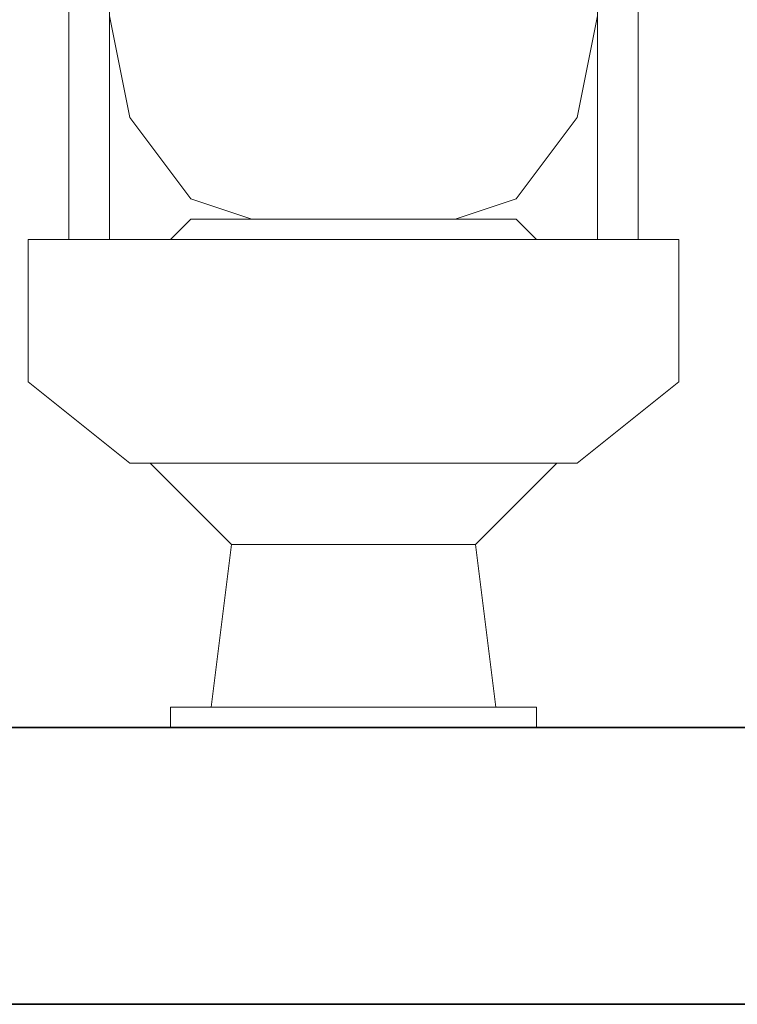
# Model space of a CAD drawing. Units: inches. Extents: x 64 to 1167, y 117 to 939.
# Tile 33 of 56: x 1051 to 1074, y 428 to 460. Entities that reach past the tile are written whole.
import ezdxf

# ---------------------------------------------------------------- set-up
doc = ezdxf.new("R2010")
doc.units = ezdxf.units.IN
doc.header["$MEASUREMENT"] = 0
doc.layers.add('A-FLOR-FIXT', color=8, linetype='Continuous', lineweight=18)
doc.layers.add('A-SECT', color=7, linetype='Continuous', lineweight=35)

# ---------------------------------------------------------------- blocks, each defined once
blk = doc.blocks.new('A$C02040E19')
for p, q in [((33.6, 403.2, 10), (33.6, 789.6, 10)), ((33.6, 403.2, 10), (33.6, 789.6, 10)), ((67.2, 789.6, 10), (67.2, 403.2, 10)), ((470.4, 789.6, 10), (470.4, 403.2, 10)), ((504, 789.6, 10), (504, 403.2, 10)), ((504, 789.6, 10), (504, 403.2, 10)), ((84, 504, 10), (67.2, 588, 10)), ((84, 504, 10), (67.2, 588, 10)), ((470.4, 588, 10), (453.6, 504, 10)), ((470.4, 588, 10), (453.6, 504, 10)), ((134.4, 436.8, 10), (84, 504, 10)), ((134.4, 436.8, 10), (84, 504, 10)), ((453.6, 504, 10), (403.2, 436.8, 10)), ((403.2, 436.8, 10), (453.6, 504, 10)), ((184.8, 420, 10), (134.4, 436.8, 10)), ((134.4, 436.8, 10), (184.8, 420, 10)), ((403.2, 436.8, 10), (352.8, 420, 10)), ((403.2, 436.8, 10), (352.8, 420, 10)), ((117.6, 403.2, 10), (134.4, 420, 10)), ((134.4, 420, 10), (117.6, 403.2, 10)), ((151.2, 420, 10), (134.4, 420, 10)), ((151.2, 420, 10), (134.4, 420, 10)), ((151.2, 420, 10), (168, 420, 10)), ((168, 420, 10), (151.2, 420, 10)), ((201.6, 420, 10), (168, 420, 10)), ((201.6, 420, 10), (168, 420, 10)), ((201.6, 420, 10), (235.2, 420, 10)), ((201.6, 420, 10), (235.2, 420, 10)), ((268.8, 420, 10), (235.2, 420, 10)), ((268.8, 420, 10), (235.2, 420, 10)), ((268.8, 420, 10), (319.2, 420, 10)), ((268.8, 420, 10), (319.2, 420, 10)), ((336, 420, 10), (319.2, 420, 10)), ((336, 420, 10), (319.2, 420, 10)), ((336, 420, 10), (369.6, 420, 10)), ((369.6, 420, 10), (336, 420, 10)), ((386.4, 420, 10), (369.6, 420, 10)), ((386.4, 420, 10), (369.6, 420, 10)), ((386.4, 420, 10), (403.2, 420, 10)), ((403.2, 420, 10), (386.4, 420, 10)), ((403.2, 420, 10), (420, 403.2, 10)), ((420, 403.2, 10), (403.2, 420, 10)), ((0, 403.2, 10), (0, 285.6, 10)), ((0, 403.2, 10), (33.6, 403.2, 10)), ((33.6, 403.2, 10), (504, 403.2, 10)), ((504, 403.2, 10), (537.6, 403.2, 10)), ((537.6, 403.2, 10), (537.6, 285.6, 10)), ((84, 218.4, 10), (0, 285.6, 10)), ((537.6, 285.6, 10), (453.6, 218.4, 10)), ((100.8, 218.4, 10), (84, 218.4, 10)), ((168, 151.2, 10), (100.8, 218.4, 10)), ((100.8, 218.4, 10), (436.8, 218.4, 10)), ((436.8, 218.4, 10), (369.6, 151.2, 10)), ((436.8, 218.4, 10), (453.6, 218.4, 10)), ((151.2, 16.8, 10), (168, 151.2, 10)), ((168, 151.2, 10), (369.6, 151.2, 10)), ((369.6, 151.2, 10), (386.4, 16.8, 10)), ((151.2, 16.8, 10), (117.6, 16.8, 10)), ((117.6, 0, 10), (117.6, 16.8, 10)), ((151.2, 16.8, 10), (386.4, 16.8, 10)), ((386.4, 16.8, 10), (420, 16.8, 10)), ((420, 16.8, 10), (420, 0, 10)), ((117.6, 0, 10), (420, 0, 10))]:
    blk.add_line(p, q)

msp = doc.modelspace()

# ---------------------------------------------------------------- linework, layer by layer
at = {"layer": 'A-SECT'}
msp.add_line((991.813, 436.679), (1157.813, 436.679), dxfattribs=at)
msp.add_lwpolyline([(982.813, 427.679), (1166.813, 427.679), (1166.813, 565.679), (982.813, 565.679)], close=True, dxfattribs=at)

# ---------------------------------------------------------------- block references
at = {"layer": 'A-FLOR-FIXT', "xscale": 0.0393700787401575, "yscale": 0.0393700787401575, "zscale": 0.0393700787401575}
msp.add_blockref('A$C02040E19', (1051.087, 436.679, -0.394), dxfattribs=at)

doc.saveas('drawing.dxf')
